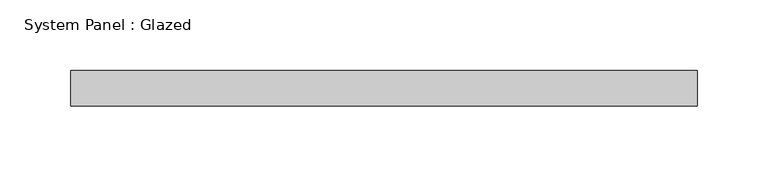
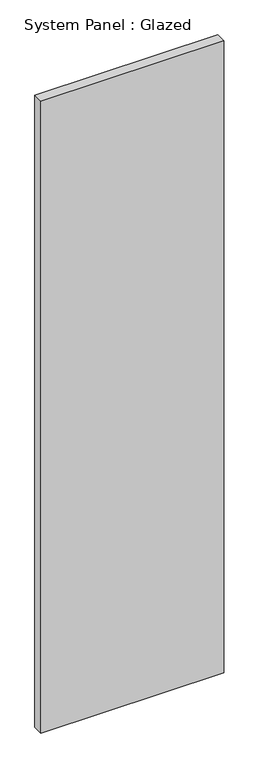
"""IFC4 building model written with IfcOpenShell, lengths in millimetres: plate geometry, System Panel : Glazed."""

from ifc_helpers import new_model, si_unit, origin, origin_with_axes, place, context, project, spatial, polyline, outline, extrude, source, transform, mapped, element, save


def system_panel_glazed_676e31df(model_context):
    return source(origin(), model_context, "Body", "SweptSolid", [
        extrude(outline(polyline([(222.25, 19.05), (-222.25, 19.05), (-222.25, 44.45), (222.25, 44.45), (222.25, 19.05)])), origin_with_axes(), (0.0, 0.0, 1.0), 1623.3622634),
    ])


if __name__ == "__main__":
    model = new_model("IFC4")
    model_context = context("Model", 3, world=origin())
    ifc_project = project(units=[si_unit("LENGTHUNIT", "METRE", prefix="MILLI")], contexts=[model_context])
    site = spatial("IfcSite", under=ifc_project)
    building = spatial("IfcBuilding", under=site)
    placement = place(None, origin())
    system_panel_glazed_shape = system_panel_glazed_676e31df(model_context)
    element("IfcPlate", 1, ObjectType="System Panel : Glazed", at=placement, inside=building, context=model_context, shape_type="MappedRepresentation", body=[
        mapped(system_panel_glazed_shape, transform((0.0, 0.0, 0.0), x_axis=(1.0, 0.0, 0.0), y_axis=(0.0, 1.0, 0.0), z_axis=(0.0, 0.0, 1.0))),
    ])
    save(model, "model.ifc")

# Revit data of these elements
# Type "System Panel : Glazed"
#   Construction Type Id = "GSP4R"
#   Analytic Construction = "1/8 in Pilkington single glazing"
#   Visual Light Transmittance = 0.9
#   Solar Heat Gain Coefficient = 0.86
#   Heat Transfer Coefficient (U) = 1.18115 BTU/(h·ft²·°F)
#   Define Thermal Properties by = 1
# Element 1 (IfcPlate, "System Panel : Glazed")
#   Materials on its faces: "Glass"
# Materials
#   "Glass": class "Glass", colour RGB 0 128 192, transparency 0.75, Description = "Soda Lime Glass", Cost = 0
